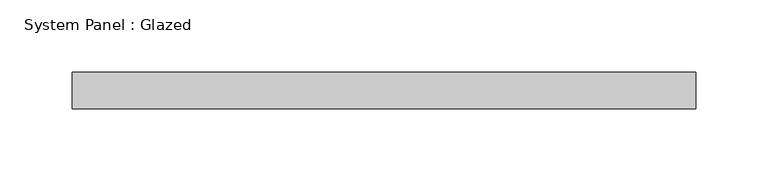
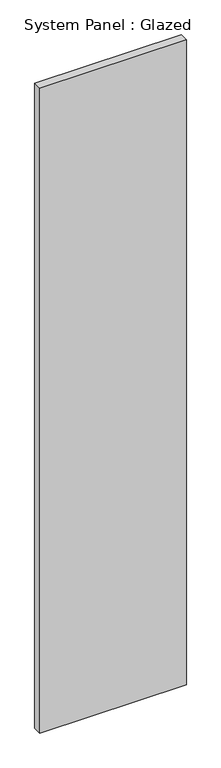
"""IFC4 building model written with IfcOpenShell, lengths in millimetres: plate geometry, System Panel : Glazed."""

from ifc_helpers import new_model, si_unit, origin, origin_with_axes, place, context, project, spatial, polyline, outline, extrude, source, transform, mapped, element, save


def system_panel_glazed_0a3516e8(model_context):
    return source(origin(), model_context, "Body", "SweptSolid", [
        extrude(outline(polyline([(215.9, -44.45), (-215.9, -44.45), (-215.9, -19.05), (215.9, -19.05), (215.9, -44.45)])), origin_with_axes(), (0.0, 0.0, 1.0), 2006.6),
    ])


if __name__ == "__main__":
    model = new_model("IFC4")
    model_context = context("Model", 3, world=origin())
    ifc_project = project(units=[si_unit("LENGTHUNIT", "METRE", prefix="MILLI")], contexts=[model_context])
    site = spatial("IfcSite", under=ifc_project)
    building = spatial("IfcBuilding", under=site)
    placement = place(None, origin())
    system_panel_glazed_shape = system_panel_glazed_0a3516e8(model_context)
    element("IfcPlate", 1, ObjectType="System Panel : Glazed", at=placement, inside=building, context=model_context, shape_type="MappedRepresentation", body=[
        mapped(system_panel_glazed_shape, transform((0.0, 0.0, 0.0), x_axis=(1.0, 0.0, 0.0), y_axis=(0.0, 1.0, 0.0), z_axis=(0.0, 0.0, 1.0))),
    ])
    save(model, "model.ifc")

# Revit data of these elements
# Type "System Panel : Glazed"
#   Construction Type Id = "GSP4R"
#   Analytic Construction = "1/8 in Pilkington single glazing"
#   Visual Light Transmittance = 0.9
#   Solar Heat Gain Coefficient = 0.86
#   Heat Transfer Coefficient (U) = 1.18115 BTU/(h·ft²·°F)
#   Define Thermal Properties by = 1
# Element 1 (IfcPlate, "System Panel : Glazed")
#   Materials on its faces: "Glass"
# Materials
#   "Glass": class "Glass", colour RGB 0 128 192, transparency 0.75, Description = "Soda Lime Glass", Cost = 0
